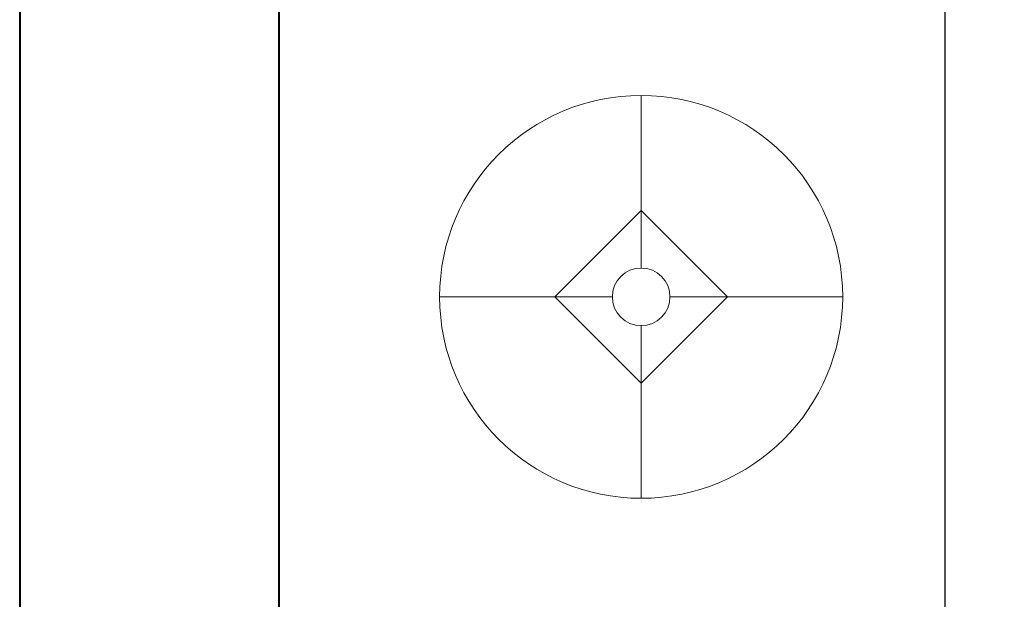
# Model space of a CAD drawing. Units: inches. Extents: x -301 to 715, y -607 to 364.
# Tile 74 of 141: x -205 to -170, y 26 to 47. Entities that reach past the tile are written whole.
import ezdxf

# ---------------------------------------------------------------- set-up
doc = ezdxf.new("R2010")
doc.units = ezdxf.units.IN
doc.header["$MEASUREMENT"] = 0
for name, color, linetype, lineweight in [('A-ANNO-DIMS', 2, 'Continuous', 18), ('A-FURN', 8, 'Continuous', 18), ('A-WALL', 3, 'Continuous', 40)]:
    doc.layers.add(name, color=color, linetype=linetype, lineweight=lineweight)
doc.styles.get("Standard").update_dxf_attribs({"font": 'arial.ttf'})
doc.dimstyles.get("Standard").update_dxf_attribs({"dimtxt": 0.18, "dimasz": 0.18, "dimexe": 0.18, "dimexo": 0.0625, "dimgap": 0.09, "dimtad": 0, "dimtih": 1, "dimtoh": 1, "dimdec": 1, "dimzin": 0, "dimdsep": 46, "dimlunit": 4, "dimtxsty": 'Standard', "dimcen": 0.09, "dimclrd": 3, "dimclre": 4, "dimclrt": 6, "dimadec": 0, "dimazin": 0, "dimtfac": 1, "dimtdec": 1, "dimtofl": 0, "dimtmove": 0, "dimatfit": 3, "dimfxl": 1, "dimtfill": 2, "dimtfillclr": 51, "dimtolj": 1, "dimtzin": 0, "dimarcsym": 0})

# ---------------------------------------------------------------- blocks, each defined once
blk = doc.blocks.new('Lamp - Table')
for p, q in [((0, 7), (0, 1)), ((0, 3), (-3, 0)), ((3, 0), (0, 3)), ((-1, 0), (-7, 0)), ((-3, 0), (0, -3)), ((0, -3), (3, 0)), ((1, 0), (7, 0)), ((0, -1), (0, -7))]:
    blk.add_line(p, q)
for radius in [7, 1]:
    blk.add_circle((0, 0), radius)
blk = doc.blocks.new('*D56')
at = {"layer": 'A-ANNO-DIMS', "color": 0, "lineweight": -2, "transparency": 16777216}
for p, q in [((-195.541, 65.682), (-172.295, 65.682)), ((-172.475, 60.682), (-172.475, 0.778)), ((-172.475, -62.318), (-172.475, -2.414)), ((-195.541, -67.318), (-172.295, -67.318))]:
    blk.add_line(p, q, dxfattribs=at)
at = {"layer": 'A-ANNO-DIMS', "color": 0, "transparency": 16777216}
for points in [[(-173.308, 60.682), (-171.641, 60.682), (-172.475, 65.682)], [(-173.308, -62.318), (-171.641, -62.318), (-172.475, -67.318)]]:
    blk.add_solid(points, dxfattribs=at)
at = {"layer": 'Defpoints', "color": 0, "transparency": 16777216}
for p in [(-195.603, 65.682), (-172.475, 65.682), (-195.603, -67.318)]:
    blk.add_point(p, dxfattribs=at)
at = {"layer": 'A-ANNO-DIMS', "color": 0, "transparency": 16777216, "insert": (-172.475, -0.818), "char_height": 3, "attachment_point": 5, "bg_fill": 1, "box_fill_scale": 1.25, "bg_fill_color": 51, "bg_fill_transparency": 0}
blk.add_mtext('\\A1;11\'-1"', dxfattribs=at)
blk = doc.blocks.new('*D151')
at = {"layer": 'A-ANNO-DIMS', "color": 4, "lineweight": -2, "transparency": 16777216}
for p, q in [((-204.603, -223.755), (-204.603, 359.612)), ((-45.603, -214.755), (-45.603, 359.612))]:
    blk.add_line(p, q, dxfattribs=at)
at = {"layer": 'A-ANNO-DIMS', "color": 3, "lineweight": -2, "transparency": 16777216}
for p, q in [((-204.423, 359.432), (-125.494, 359.432)), ((-45.783, 359.432), (-124.713, 359.432))]:
    blk.add_line(p, q, dxfattribs=at)
at = {"layer": 'A-ANNO-DIMS', "color": 3, "transparency": 16777216}
for points in [[(-204.423, 359.462), (-204.423, 359.402), (-204.603, 359.432)], [(-45.783, 359.462), (-45.783, 359.402), (-45.603, 359.432)]]:
    blk.add_solid(points, dxfattribs=at)
at = {"layer": 'Defpoints', "color": 0, "transparency": 16777216}
for p in [(-45.603, 359.432), (-45.603, -214.818), (-204.603, -223.818)]:
    blk.add_point(p, dxfattribs=at)
at = {"layer": 'A-ANNO-DIMS', "color": 6, "transparency": 16777216, "insert": (-125.103, 359.432), "char_height": 0.18, "attachment_point": 5, "bg_fill": 1, "box_fill_scale": 1.25, "bg_fill_color": 51, "bg_fill_transparency": 0}
blk.add_mtext('\\A1;13\'-3"', dxfattribs=at)

msp = doc.modelspace()

# ---------------------------------------------------------------- linework, layer by layer
at = {"layer": 'A-WALL'}
for p, q in [((-204.603, 71.682), (-204.603, -67.318)), ((-195.603, 65.682), (-195.603, -67.318))]:
    msp.add_line(p, q, dxfattribs=at)

# ---------------------------------------------------------------- block references
at = {"layer": 'A-FURN'}
msp.add_blockref('Lamp - Table', (-183.017, 36.891), dxfattribs=at)

# ---------------------------------------------------------------- dimensions: what is measured, and where the dimension line sits
at = {"layer": 'A-ANNO-DIMS'}
dim = msp.add_linear_dim(base=(-45.603, 359.432), p1=(-204.603, -223.818), p2=(-45.603, -214.818), dimstyle='Standard', override={"dimdec": 1, "dimlfac": 1, "dimrnd": 0, "dimzin": 1, "dimdsep": 46, "dimlunit": 4, "dimfrac": 2}, dxfattribs=at)
dim.commit()
dim.dimension.update_dxf_attribs({"geometry": '*D151', "text_midpoint": (-125.103, 359.432)})
dim = msp.add_linear_dim(base=(-172.475, 65.682), p1=(-195.603, -67.318), p2=(-195.603, 65.682), angle=90, dimstyle='Standard', override={"dimtxt": 3, "dimasz": 5, "dimclrd": 0, "dimclre": 0, "dimclrt": 0}, dxfattribs=at)
dim.commit()
dim.dimension.update_dxf_attribs({"geometry": '*D56', "text_midpoint": (-172.475, -0.818)})

doc.saveas('drawing.dxf')
